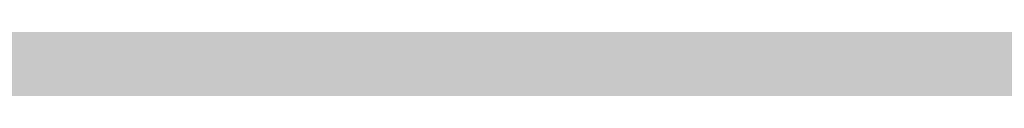
# Model space of a CAD drawing. Units: millimetres. Extents: x 0 to 2267, y 0 to 1823.
# Tile 100 of 256: x 1600.369 to 1605.705, y 1227.466 to 1227.736. Entities that reach past the tile are written whole.
import ezdxf

# ---------------------------------------------------------------- set-up
doc = ezdxf.new("R2010")
doc.units = ezdxf.units.MM
doc.header["$MEASUREMENT"] = 0
doc.layers.add('M-DIMS', color=2, linetype='Continuous', lineweight=25)
doc.layers.add('M-HATC', color=252, linetype='Continuous', lineweight=18)
doc.styles.get("Standard").update_dxf_attribs({"font": 'arial.ttf'})
doc.dimstyles.get("Standard").update_dxf_attribs({"dimtxt": 7, "dimasz": 4, "dimexe": 0.18, "dimexo": 0.0625, "dimgap": 0.09, "dimtad": 0, "dimdec": 0, "dimzin": 0, "dimdsep": 46, "dimtxsty": 'Standard', "dimcen": 0.09, "dimadec": 0, "dimazin": 0, "dimtfac": 1, "dimtdec": 0, "dimtofl": 0, "dimtmove": 0, "dimatfit": 3, "dimfxl": 1, "dimtolj": 1, "dimtzin": 0, "dimarcsym": 0})

# ---------------------------------------------------------------- blocks, each defined once
blk = doc.blocks.new('*D19')
at = {"layer": 'Defpoints', "color": 0, "transparency": 16777216}
for p in [(1605.3399, 1483.3044), (1445.5291, 1333.8851)]:
    blk.add_point(p, dxfattribs=at)
at = {"layer": 'M-DIMS', "color": 0, "lineweight": -2, "transparency": 16777216}
for p, q in [((1605.3399, 1483.2144), (1605.3399, 1483.3944)), ((1605.2499, 1483.3044), (1605.4299, 1483.3044)), ((1366.3244, 1259.8306), (1442.6072, 1331.1532))]:
    blk.add_line(p, q, dxfattribs=at)
at = {"layer": 'M-DIMS', "color": 0, "transparency": 16777216}
blk.add_solid([(1442.1519, 1331.6402), (1443.0625, 1330.6663), (1445.5291, 1333.8851)], dxfattribs=at)
at = {"layer": 'M-DIMS', "color": 0, "transparency": 16777216, "insert": (1349.6425, 1244.2335), "char_height": 7, "attachment_point": 5, "rotation": 43.0753}
blk.add_mtext('\\A1;2X R218.8', dxfattribs=at)

msp = doc.modelspace()

# ---------------------------------------------------------------- hatches: boundary and pattern name
at = {"layer": 'M-HATC'}
h = msp.add_hatch(color=256, dxfattribs=at)
h.dxf.hatch_style = 1
h.paths.add_polyline_path([(2055.771, 1603.062), (1381.0868, 1603.062), (1381.0868, 1598.062), (2055.771, 1598.062)])
h.paths.add_polyline_path([(2055.771, 1598.062), (1381.0868, 1598.062), (1381.0868, 1593.062), (2055.771, 1593.062)])
h.paths.add_polyline_path([(2051.3074, 1536.7609), (1385.5504, 1536.7609), (1385.5504, 1526.7609), (1387.5504, 1526.7609), (1388.5366, 1525.0528), (1385.3319, 1521.2335), (1385.3319, 1521.2226), (2050.2542, 1522.7491), (2048.3212, 1525.0528), (2049.3074, 1526.7609), (2051.3074, 1526.7609)])
edge = h.paths.add_edge_path()
edge.add_arc((1847.5345, 1379.1492), 135, 222.603061, 222.890851, ccw=False)
edge.add_line((1748.1663, 1287.7656), (1683.0921, 1287.7656))
edge.add_arc((1583.7239, 1379.1492), 135, 317.109149, 317.396939, ccw=False)
edge.add_arc((1678.9686, 1290.6707), 5, 222.8909, 317.1091, ccw=False)
edge.add_arc((1774.2133, 1379.1492), 135, 222.603061, 222.890851, ccw=False)
edge.add_line((1674.8451, 1287.7656), (1609.7709, 1287.7656))
edge.add_arc((1510.4027, 1379.1492), 135, 317.109149, 317.396939, ccw=False)
edge.add_arc((1605.6474, 1290.6707), 5, 222.8909, 317.1091, ccw=False)
edge.add_arc((1700.8921, 1379.1492), 135, 222.603061, 222.890851, ccw=False)
edge.add_line((1601.5239, 1287.7656), (1536.4497, 1287.7656))
edge.add_arc((1437.0815, 1379.1492), 135, 317.109149, 317.396939, ccw=False)
edge.add_arc((1532.3262, 1290.6707), 5, 222.8909, 317.1091, ccw=False)
edge.add_arc((1627.5709, 1379.1492), 135, 222.603061, 222.890851, ccw=False)
edge.add_line((1528.2027, 1287.7656), (1505.9289, 1287.7656))
edge.add_spline(control_points=[(1505.9289, 1287.7656), (1504.2622, 1287.7656), (1504.2622, 1282.7656), (1505.9289, 1282.7656)], knot_values=[0, 0, 0, 0, 5, 5, 5, 5], degree=3, periodic=0)
edge.add_line((1505.9289, 1282.7656), (1930.9289, 1282.7656))
edge.add_spline(control_points=[(1930.9289, 1282.7656), (1932.5956, 1282.7656), (1932.5956, 1287.7656), (1930.9289, 1287.7656)], knot_values=[0, 0, 0, 0, 5, 5, 5, 5], degree=3, periodic=0)
edge.add_line((1930.9289, 1287.7656), (1903.0557, 1287.7656))
edge.add_arc((1803.6875, 1379.1492), 135, 317.109149, 317.396939, ccw=False)
edge.add_arc((1898.9322, 1290.6707), 5, 222.8909, 317.1091, ccw=False)
edge.add_arc((1994.1769, 1379.1492), 135, 222.603061, 222.890851, ccw=False)
edge.add_line((1894.8087, 1287.7656), (1829.7345, 1287.7656))
edge.add_arc((1730.3663, 1379.1492), 135, 317.109149, 317.396939, ccw=False)
edge.add_arc((1825.611, 1290.6707), 5, 222.8909, 317.1091, ccw=False)
edge.add_arc((1920.8557, 1379.1492), 135, 222.603061, 222.890851, ccw=False)
edge.add_line((1821.4875, 1287.7656), (1756.4133, 1287.7656))
edge.add_arc((1657.0451, 1379.1492), 135, 317.109149, 317.396939, ccw=False)
edge.add_arc((1752.2898, 1290.6707), 5, 222.8909, 317.1091, ccw=False)
edge = h.paths.add_edge_path()
edge.add_spline(control_points=[(1843.4289, 1227.2475), (1845.0956, 1227.2475), (1845.0956, 1232.2475), (1843.4289, 1232.2475)], knot_values=[0, 0, 0, 0, 5, 5, 5, 5], degree=3, periodic=0)
edge.add_line((1843.4289, 1232.2475), (1593.4289, 1232.2475))
edge.add_spline(control_points=[(1593.4289, 1232.2475), (1591.7622, 1232.2475), (1591.7622, 1227.2475), (1593.4289, 1227.2475)], knot_values=[0, 0, 0, 0, 5, 5, 5, 5], degree=3, periodic=0)
edge.add_line((1593.4289, 1227.2475), (1843.4289, 1227.2475))
h.paths.add_polyline_path([(1905.9289, 1127.4171), (1530.9289, 1127.4171, 0.414214), (1520.9289, 1117.4171), (1530.9289, 1117.4171), (1915.9289, 1117.4171, 0.414214)])
edge = h.paths.add_edge_path()
edge.add_arc((1397.0858, 1498.4078), 12.7299, 90.78215, 190.87871, ccw=False)
edge.add_line((1396.912, 1511.1365), (1428.0097, 1511.3488))
edge.add_line((1428.0097, 1511.3488), (1433.0097, 1511.3488))
edge.add_line((1433.0097, 1511.3488), (1434.439, 1511.3488))
edge.add_arc((1419.474, 1498.0804), 20, 41.561, 74.08211)
edge.add_line((1424.9592, 1517.3135), (1399.9351, 1517.2561))
edge.add_spline(control_points=[(1399.9307, 1517.2561), (1399.884, 1517.2131), (1399.8328, 1517.1689), (1399.7774, 1517.1236)], knot_values=[11.567499, 11.567499, 11.567499, 11.567499, 11.814249, 11.814249, 11.814249, 11.814249], degree=3, periodic=0)
edge.add_spline(control_points=[(1399.6328, 1517.0099), (1399.5831, 1516.9721), (1399.5307, 1516.9338), (1399.4759, 1516.8947)], knot_values=[11.167718, 11.167718, 11.167718, 11.167718, 11.365188, 11.365188, 11.365188, 11.365188], degree=3, periodic=0)
edge.add_spline(control_points=[(1399.3398, 1516.8001), (1399.1514, 1516.6719), (1398.9384, 1516.5377), (1398.704, 1516.3994)], knot_values=[10.376405, 10.376405, 10.376405, 10.376405, 11.00994, 11.00994, 11.00994, 11.00994], degree=3, periodic=0)
edge.add_spline(control_points=[(1398.6572, 1516.3719), (1398.5789, 1516.326), (1398.4983, 1516.2797), (1398.4155, 1516.2331)], knot_values=[10.125175, 10.125175, 10.125175, 10.125175, 10.334406, 10.334406, 10.334406, 10.334406], degree=3, periodic=0)
edge.add_spline(control_points=[(1398.2642, 1516.1487), (1398.196, 1516.1111), (1398.1263, 1516.0732), (1398.0555, 1516.0351)], knot_values=[9.832246, 9.832246, 9.832246, 9.832246, 9.999658, 9.999658, 9.999658, 9.999658], degree=3, periodic=0)
edge.add_spline(control_points=[(1397.9987, 1516.0048), (1397.7312, 1515.8621), (1397.446, 1515.7171), (1397.1466, 1515.5714)], knot_values=[9.161808, 9.161808, 9.161808, 9.161808, 9.787769, 9.787769, 9.787769, 9.787769], degree=3, periodic=0)
edge.add_spline(control_points=[(1397.1466, 1515.5714), (1396.8418, 1515.423), (1396.5222, 1515.274), (1396.1914, 1515.1262)], knot_values=[8.524455, 8.524455, 8.524455, 8.524455, 9.161808, 9.161808, 9.161808, 9.161808], degree=3, periodic=0)
edge.add_spline(control_points=[(1396.0777, 1515.0756), (1395.9854, 1515.0348), (1395.8922, 1514.994), (1395.7983, 1514.9534)], knot_values=[8.275193, 8.275193, 8.275193, 8.275193, 8.451726, 8.451726, 8.451726, 8.451726], degree=3, periodic=0)
edge.add_spline(control_points=[(1395.6018, 1514.8691), (1395.4997, 1514.8257), (1395.3968, 1514.7824), (1395.2932, 1514.7394)], knot_values=[7.962917, 7.962917, 7.962917, 7.962917, 8.152764, 8.152764, 8.152764, 8.152764], degree=3, periodic=0)
edge.add_spline(control_points=[(1395.2116, 1514.7057), (1394.8278, 1514.5475), (1394.4345, 1514.3929), (1394.0364, 1514.2442)], knot_values=[7.21254, 7.21254, 7.21254, 7.21254, 7.913148, 7.913148, 7.913148, 7.913148], degree=3, periodic=0)
edge.add_spline(control_points=[(1394.0364, 1514.2442), (1393.7076, 1514.1214), (1393.3754, 1514.0027), (1393.0427, 1513.8895)], knot_values=[6.633733, 6.633733, 6.633733, 6.633733, 7.21254, 7.21254, 7.21254, 7.21254], degree=3, periodic=0)
edge.add_spline(control_points=[(1392.8214, 1513.815), (1392.7198, 1513.7812), (1392.6181, 1513.7479), (1392.5166, 1513.7152)], knot_values=[6.328796, 6.328796, 6.328796, 6.328796, 6.505493, 6.505493, 6.505493, 6.505493], degree=3, periodic=0)
edge.add_spline(control_points=[(1392.5166, 1513.7152), (1392.3187, 1513.6515), (1392.1212, 1513.59), (1391.9244, 1513.531)], knot_values=[5.984605, 5.984605, 5.984605, 5.984605, 6.328796, 6.328796, 6.328796, 6.328796], degree=3, periodic=0)
edge.add_spline(control_points=[(1391.7915, 1513.4915), (1391.3122, 1513.3501), (1390.8384, 1513.2239), (1390.3784, 1513.1171)], knot_values=[5.066697, 5.066697, 5.066697, 5.066697, 5.907055, 5.907055, 5.907055, 5.907055], degree=3, periodic=0)
edge.add_spline(control_points=[(1390.3784, 1513.1171), (1390.1797, 1513.071), (1389.9836, 1513.0284), (1389.7907, 1512.9899)], knot_values=[4.70367, 4.70367, 4.70367, 4.70367, 5.066695, 5.066695, 5.066695, 5.066695], degree=3, periodic=0)
edge.add_spline(control_points=[(1389.422, 1512.9204), (1389.2459, 1512.8892), (1389.0729, 1512.8617), (1388.9036, 1512.8381)], knot_values=[4.130571, 4.130571, 4.130571, 4.130571, 4.469816, 4.469816, 4.469816, 4.469816], degree=3, periodic=0)
edge.add_spline(control_points=[(1388.9036, 1512.8381), (1388.591, 1512.7946), (1388.2911, 1512.7644), (1388.0071, 1512.7494)], knot_values=[3.504031, 3.504031, 3.504031, 3.504031, 4.130571, 4.130571, 4.130571, 4.130571], degree=3, periodic=0)
edge.add_spline(control_points=[(1387.9356, 1512.7459), (1387.8538, 1512.7423), (1387.7733, 1512.74), (1387.6944, 1512.739)], knot_values=[3.268866, 3.268866, 3.268866, 3.268866, 3.451164, 3.451164, 3.451164, 3.451164], degree=3, periodic=0)
edge.add_spline(control_points=[(1387.3351, 1512.7443), (1387.2076, 1512.7499), (1387.0847, 1512.7597), (1386.967, 1512.7739)], knot_values=[2.670686, 2.670686, 2.670686, 2.670686, 2.984, 2.984, 2.984, 2.984], degree=3, periodic=0)
edge.add_spline(control_points=[(1386.8327, 1512.7922), (1386.8209, 1512.7941), (1386.8092, 1512.7959), (1386.7975, 1512.7979)], knot_values=[2.516981, 2.516981, 2.516981, 2.516981, 2.549528, 2.549528, 2.549528, 2.549528], degree=3, periodic=0)
edge.add_spline(control_points=[(1386.4526, 1512.8735), (1386.4257, 1512.881), (1386.3993, 1512.889), (1386.3733, 1512.8972)], knot_values=[2.095869, 2.095869, 2.095869, 2.095869, 2.17941, 2.17941, 2.17941, 2.17941], degree=3, periodic=0)
edge.add_spline(control_points=[(1386.0691, 1513.0189), (1386.0634, 1513.0217), (1386.0577, 1513.0246), (1386.052, 1513.0275)], knot_values=[1.72453, 1.72453, 1.72453, 1.72453, 1.745933, 1.745933, 1.745933, 1.745933], degree=3, periodic=0)
edge.add_arc((1399.474, 1498.0804), 20, 131.82432, 180)
edge.add_arc((1630.3336, 1505.5484), 250.9708, 181.705176, 236.427975)
edge.add_arc((1605.3399, 1483.3044), 218.7822, 238.660829, 243.34961)
edge.add_arc((1647.0911, 1510.3592), 262.8986, 183.129836, 237.853442, ccw=False)
h.paths.add_polyline_path([(1406.5369, 1391.9644, 0.149382), (1491.5506, 1296.4418, -0.129517)], flags=17)
edge = h.paths.add_edge_path()
edge.add_arc((2037.3838, 1498.0804), 20, 0, 48.26587)
edge.add_spline(control_points=[(2050.6973, 1513.0052), (2050.6512, 1512.9847), (2050.6034, 1512.9655), (2050.5539, 1512.9477)], knot_values=[1.835652, 1.835652, 1.835652, 1.835652, 2.000781, 2.000781, 2.000781, 2.000781], degree=3, periodic=0)
edge.add_spline(control_points=[(2050.4616, 1512.9166), (2050.479, 1512.9221), (2050.4963, 1512.9277), (2050.5133, 1512.9335)], knot_values=[2.045477, 2.045477, 2.045477, 2.045477, 2.101389, 2.101389, 2.101389, 2.101389], degree=3, periodic=0)
edge.add_spline(control_points=[(2050.129, 1512.8342), (2050.1984, 1512.8473), (2050.2657, 1512.8623), (2050.3308, 1512.8792)], knot_values=[2.237629, 2.237629, 2.237629, 2.237629, 2.435841, 2.435841, 2.435841, 2.435841], degree=3, periodic=0)
edge.add_spline(control_points=[(2050.0946, 1512.8278), (2050.1061, 1512.8299), (2050.1176, 1512.832), (2050.129, 1512.8342)], knot_values=[2.435841, 2.435841, 2.435841, 2.435841, 2.468321, 2.468321, 2.468321, 2.468321], degree=3, periodic=0)
edge.add_spline(control_points=[(2049.7843, 1512.7851), (2049.8552, 1512.7922), (2049.9243, 1512.8008), (2049.9917, 1512.8109)], knot_values=[2.563852, 2.563852, 2.563852, 2.563852, 2.748541, 2.748541, 2.748541, 2.748541], degree=3, periodic=0)
edge.add_spline(control_points=[(2049.4052, 1512.7617), (2049.5364, 1512.7653), (2049.6629, 1512.773), (2049.7843, 1512.7851)], knot_values=[2.748541, 2.748541, 2.748541, 2.748541, 3.064882, 3.064882, 3.064882, 3.064882], degree=3, periodic=0)
edge.add_spline(control_points=[(2049.1698, 1512.7597), (2049.2336, 1512.7591), (2049.2965, 1512.7594), (2049.3584, 1512.7606)], knot_values=[3.102309, 3.102309, 3.102309, 3.102309, 3.2503, 3.2503, 3.2503, 3.2503], degree=3, periodic=0)
edge.add_spline(control_points=[(2048.8573, 1512.7691), (2048.9638, 1512.7638), (2049.068, 1512.7606), (2049.1698, 1512.7597)], knot_values=[3.2503, 3.2503, 3.2503, 3.2503, 3.486069, 3.486069, 3.486069, 3.486069], degree=3, periodic=0)
edge.add_spline(control_points=[(2048.6924, 1512.7789), (2048.3729, 1512.8009), (2048.0345, 1512.8411), (2047.6817, 1512.897)], knot_values=[3.606429, 3.606429, 3.606429, 3.606429, 4.2989, 4.2989, 4.2989, 4.2989], degree=3, periodic=0)
edge.add_spline(control_points=[(2047.6817, 1512.897), (2047.5458, 1512.9185), (2047.4077, 1512.9424), (2047.2678, 1512.9685)], knot_values=[4.2989, 4.2989, 4.2989, 4.2989, 4.565769, 4.565769, 4.565769, 4.565769], degree=3, periodic=0)
edge.add_spline(control_points=[(2047.2678, 1512.9685), (2047.1449, 1512.9914), (2047.0207, 1513.016), (2046.8951, 1513.0422)], knot_values=[4.565769, 4.565769, 4.565769, 4.565769, 4.799971, 4.799971, 4.799971, 4.799971], degree=3, periodic=0)
edge.add_spline(control_points=[(2046.8951, 1513.0422), (2046.5286, 1513.1188), (2046.1513, 1513.209), (2045.7676, 1513.3107)], knot_values=[4.799971, 4.799971, 4.799971, 4.799971, 5.483718, 5.483718, 5.483718, 5.483718], degree=3, periodic=0)
edge.add_spline(control_points=[(2045.7676, 1513.3107), (2045.3724, 1513.4154), (2044.9704, 1513.5322), (2044.5662, 1513.6588)], knot_values=[5.483718, 5.483718, 5.483718, 5.483718, 6.187866, 6.187866, 6.187866, 6.187866], degree=3, periodic=0)
edge.add_spline(control_points=[(2044.5662, 1513.6588), (2044.4149, 1513.7061), (2044.2633, 1513.7549), (2044.1116, 1513.8048)], knot_values=[6.187866, 6.187866, 6.187866, 6.187866, 6.451551, 6.451551, 6.451551, 6.451551], degree=3, periodic=0)
edge.add_spline(control_points=[(2044.1116, 1513.8048), (2043.9967, 1513.8427), (2043.8817, 1513.8813), (2043.7668, 1513.9205)], knot_values=[6.451551, 6.451551, 6.451551, 6.451551, 6.651434, 6.651434, 6.651434, 6.651434], degree=3, periodic=0)
edge.add_spline(control_points=[(2043.7668, 1513.9205), (2043.3716, 1514.0554), (2042.9774, 1514.1979), (2042.5886, 1514.3458)], knot_values=[6.651434, 6.651434, 6.651434, 6.651434, 7.338879, 7.338879, 7.338879, 7.338879], degree=3, periodic=0)
edge.add_spline(control_points=[(2042.5886, 1514.3458), (2042.1643, 1514.5071), (2041.7465, 1514.6749), (2041.3409, 1514.846)], knot_values=[7.338879, 7.338879, 7.338879, 7.338879, 8.089209, 8.089209, 8.089209, 8.089209], degree=3, periodic=0)
edge.add_spline(control_points=[(2041.3409, 1514.846), (2041.1028, 1514.9465), (2040.869, 1515.0481), (2040.6405, 1515.1502)], knot_values=[8.089209, 8.089209, 8.089209, 8.089209, 8.529587, 8.529587, 8.529587, 8.529587], degree=3, periodic=0)
edge.add_spline(control_points=[(2040.51, 1515.2089), (2040.0824, 1515.4022), (2039.6747, 1515.5971), (2039.295, 1515.7894)], knot_values=[8.613818, 8.613818, 8.613818, 8.613818, 9.44571, 9.44571, 9.44571, 9.44571], degree=3, periodic=0)
edge.add_spline(control_points=[(2039.295, 1515.7894), (2039.0618, 1515.9075), (2038.8391, 1516.0246), (2038.6288, 1516.1398)], knot_values=[9.44571, 9.44571, 9.44571, 9.44571, 9.956404, 9.956404, 9.956404, 9.956404], degree=3, periodic=0)
edge.add_spline(control_points=[(2038.6288, 1516.1398), (2038.5187, 1516.2001), (2038.4121, 1516.2598), (2038.309, 1516.3189)], knot_values=[9.956404, 9.956404, 9.956404, 9.956404, 10.223542, 10.223542, 10.223542, 10.223542], degree=3, periodic=0)
edge.add_spline(control_points=[(2038.309, 1516.3189), (2038.2138, 1516.3735), (2038.1216, 1516.4276), (2038.0328, 1516.481)], knot_values=[10.223542, 10.223542, 10.223542, 10.223542, 10.47051, 10.47051, 10.47051, 10.47051], degree=3, periodic=0)
edge.add_spline(control_points=[(2038.0328, 1516.481), (2037.7855, 1516.6296), (2037.5639, 1516.773), (2037.3722, 1516.909)], knot_values=[10.47051, 10.47051, 10.47051, 10.47051, 11.15767, 11.15767, 11.15767, 11.15767], degree=3, periodic=0)
edge.add_spline(control_points=[(2037.3722, 1516.909), (2037.2789, 1516.9752), (2037.1927, 1517.0396), (2037.1142, 1517.102)], knot_values=[11.15767, 11.15767, 11.15767, 11.15767, 11.49227, 11.49227, 11.49227, 11.49227], degree=3, periodic=0)
edge.add_spline(control_points=[(2036.8564, 1517.3259), (2036.9148, 1517.2692), (2036.9814, 1517.2103), (2037.0557, 1517.1492)], knot_values=[11.577341, 11.577341, 11.577341, 11.577341, 11.91035, 11.91035, 11.91035, 11.91035], degree=3, periodic=0)
edge.add_spline(control_points=[(2036.8074, 1517.3748), (2036.823, 1517.3587), (2036.8393, 1517.3424), (2036.8564, 1517.3259)], knot_values=[11.91035, 11.91035, 11.91035, 11.91035, 12.007402, 12.007402, 12.007402, 12.007402], degree=3, periodic=0)
edge.add_spline(control_points=[(2036.7017, 1517.494), (2036.7104, 1517.483), (2036.7196, 1517.4719), (2036.7291, 1517.4606)], knot_values=[12.184155, 12.184155, 12.184155, 12.184155, 12.255409, 12.255409, 12.255409, 12.255409], degree=3, periodic=0)
edge.add_spline(control_points=[(2036.6159, 1517.6205), (2036.62, 1517.613), (2036.6243, 1517.6055), (2036.6289, 1517.5979)], knot_values=[12.487913, 12.487913, 12.487913, 12.487913, 12.541035, 12.541035, 12.541035, 12.541035], degree=3, periodic=0)
edge.add_spline(control_points=[(2036.5635, 1517.786), (2036.5637, 1517.7794), (2036.5642, 1517.7726), (2036.565, 1517.7658)], knot_values=[12.911761, 12.911761, 12.911761, 12.911761, 12.968286, 12.968286, 12.968286, 12.968286], degree=3, periodic=0)
edge.add_spline(control_points=[(2036.6166, 1517.9304), (2036.6125, 1517.9259), (2036.6086, 1517.9212), (2036.6049, 1517.9165)], knot_values=[13.382527, 13.382527, 13.382527, 13.382527, 13.433791, 13.433791, 13.433791, 13.433791], degree=3, periodic=0)
edge.add_spline(control_points=[(2036.749, 1518.017), (2036.7361, 1518.0116), (2036.7239, 1518.006), (2036.7124, 1518.0002)], knot_values=[13.726299, 13.726299, 13.726299, 13.726299, 13.809928, 13.809928, 13.809928, 13.809928], degree=3, periodic=0)
edge.add_spline(control_points=[(2036.8604, 1518.0528), (2036.8386, 1518.0474), (2036.8181, 1518.0416), (2036.7988, 1518.0353)], knot_values=[13.910887, 13.910887, 13.910887, 13.910887, 14.02153, 14.02153, 14.02153, 14.02153], degree=3, periodic=0)
edge.add_line((2036.9639, 1518.0804), (2032.3838, 1518.0804))
edge.add_line((2032.3838, 1518.0804), (2027.3838, 1518.0804))
edge.add_line((2027.3838, 1518.0804), (2022.3838, 1518.0804))
edge.add_line((2022.3838, 1518.0804), (2017.3838, 1518.0804))
edge.add_arc((2017.3838, 1498.0804), 20, 90, 138.439)
edge.add_line((2002.4188, 1511.3488), (2003.8481, 1511.3488))
edge.add_line((2003.8481, 1511.3488), (2008.8481, 1511.3488))
edge.add_line((2008.8481, 1511.3488), (2039.772, 1511.1377))
edge.add_arc((2039.772, 1498.4078), 12.7299, -10.87871, 90, ccw=False)
edge.add_arc((1789.7668, 1510.3592), 262.8986, 302.146558, 356.870164, ccw=False)
edge.add_arc((1831.5179, 1483.3044), 218.7822, 296.65039, 301.339171)
edge.add_arc((1806.5242, 1505.5484), 250.9708, 303.572025, 358.294824)
h.paths.add_polyline_path([(2030.321, 1391.9644, -0.129517), (1945.3072, 1296.4418, 0.149382)], flags=17)
edge = h.paths.add_edge_path()
edge.add_spline(control_points=[(2037.2464, 1518.0821), (2037.2898, 1518.081), (2037.3355, 1518.0804), (2037.3838, 1518.0804)], knot_values=[0.000012, 0.000012, 0.000012, 0.000012, 0.144754, 0.144754, 0.144754, 0.144754], degree=3, periodic=0)
edge.add_line((2037.3357, 1518.0804), (2037.0096, 1518.0804))
edge.add_spline(control_points=[(2037.0096, 1518.0804), (2036.9822, 1518.0768), (2036.956, 1518.0727), (2036.9312, 1518.0681)], knot_values=[14.13465, 14.13465, 14.13465, 14.13465, 14.247197, 14.247197, 14.247197, 14.247197], degree=3, periodic=0)
edge.add_spline(control_points=[(2036.9312, 1518.0681), (2036.9276, 1518.0674), (2036.9241, 1518.0667), (2036.9205, 1518.0661)], knot_values=[14.118315, 14.118315, 14.118315, 14.118315, 14.13465, 14.13465, 14.13465, 14.13465], degree=3, periodic=0)
edge.add_spline(control_points=[(2036.9205, 1518.0661), (2036.9118, 1518.0644), (2036.9032, 1518.0626), (2036.8948, 1518.0608)], knot_values=[14.078086, 14.078086, 14.078086, 14.078086, 14.118315, 14.118315, 14.118315, 14.118315], degree=3, periodic=0)
edge.add_spline(control_points=[(2036.8948, 1518.0608), (2036.883, 1518.0583), (2036.8716, 1518.0556), (2036.8604, 1518.0528)], knot_values=[14.02153, 14.02153, 14.02153, 14.02153, 14.078086, 14.078086, 14.078086, 14.078086], degree=3, periodic=0)
edge.add_spline(control_points=[(2036.8604, 1518.0528), (2036.8386, 1518.0474), (2036.8181, 1518.0416), (2036.7988, 1518.0353)], knot_values=[13.910887, 13.910887, 13.910887, 13.910887, 14.02153, 14.02153, 14.02153, 14.02153], degree=3, periodic=0)
edge.add_spline(control_points=[(2036.7988, 1518.0353), (2036.7981, 1518.035), (2036.7974, 1518.0348), (2036.7967, 1518.0346)], knot_values=[13.906906, 13.906906, 13.906906, 13.906906, 13.910887, 13.910887, 13.910887, 13.910887], degree=3, periodic=0)
edge.add_spline(control_points=[(2036.7967, 1518.0346), (2036.7882, 1518.0318), (2036.7799, 1518.0289), (2036.7719, 1518.0259)], knot_values=[13.857826, 13.857826, 13.857826, 13.857826, 13.906906, 13.906906, 13.906906, 13.906906], degree=3, periodic=0)
edge.add_spline(control_points=[(2036.7719, 1518.0259), (2036.764, 1518.023), (2036.7564, 1518.02), (2036.749, 1518.017)], knot_values=[13.809928, 13.809928, 13.809928, 13.809928, 13.857826, 13.857826, 13.857826, 13.857826], degree=3, periodic=0)
edge.add_spline(control_points=[(2036.749, 1518.017), (2036.7361, 1518.0116), (2036.7239, 1518.006), (2036.7124, 1518.0002)], knot_values=[13.726299, 13.726299, 13.726299, 13.726299, 13.809928, 13.809928, 13.809928, 13.809928], degree=3, periodic=0)
edge.add_spline(control_points=[(2036.7124, 1518.0002), (2036.7121, 1518), (2036.7118, 1517.9999), (2036.7115, 1517.9997)], knot_values=[13.723993, 13.723993, 13.723993, 13.723993, 13.726299, 13.726299, 13.726299, 13.726299], degree=3, periodic=0)
edge.add_spline(control_points=[(2036.7115, 1517.9997), (2036.7063, 1517.9971), (2036.7013, 1517.9944), (2036.6965, 1517.9917)], knot_values=[13.686536, 13.686536, 13.686536, 13.686536, 13.723993, 13.723993, 13.723993, 13.723993], degree=3, periodic=0)
edge.add_spline(control_points=[(2036.6965, 1517.9917), (2036.6919, 1517.9891), (2036.6874, 1517.9865), (2036.6831, 1517.9839)], knot_values=[13.651251, 13.651251, 13.651251, 13.651251, 13.686536, 13.686536, 13.686536, 13.686536], degree=3, periodic=0)
edge.add_spline(control_points=[(2036.6831, 1517.9839), (2036.6764, 1517.9798), (2036.67, 1517.9757), (2036.6639, 1517.9714)], knot_values=[13.596804, 13.596804, 13.596804, 13.596804, 13.651251, 13.651251, 13.651251, 13.651251], degree=3, periodic=0)
edge.add_spline(control_points=[(2036.6639, 1517.9714), (2036.6636, 1517.9712), (2036.6633, 1517.9709), (2036.6629, 1517.9707)], knot_values=[13.593956, 13.593956, 13.593956, 13.593956, 13.596804, 13.596804, 13.596804, 13.596804], degree=3, periodic=0)
edge.add_spline(control_points=[(2036.6629, 1517.9707), (2036.6603, 1517.9689), (2036.6577, 1517.967), (2036.6552, 1517.9651)], knot_values=[13.570322, 13.570322, 13.570322, 13.570322, 13.593956, 13.593956, 13.593956, 13.593956], degree=3, periodic=0)
edge.add_spline(control_points=[(2036.6552, 1517.9651), (2036.6525, 1517.9631), (2036.6499, 1517.9611), (2036.6474, 1517.9591)], knot_values=[13.545477, 13.545477, 13.545477, 13.545477, 13.570322, 13.570322, 13.570322, 13.570322], degree=3, periodic=0)
edge.add_spline(control_points=[(2036.6474, 1517.9591), (2036.6472, 1517.9589), (2036.6471, 1517.9588), (2036.6469, 1517.9587)], knot_values=[13.543931, 13.543931, 13.543931, 13.543931, 13.545477, 13.545477, 13.545477, 13.545477], degree=3, periodic=0)
edge.add_spline(control_points=[(2036.6469, 1517.9587), (2036.6412, 1517.9541), (2036.6358, 1517.9494), (2036.6307, 1517.9447)], knot_values=[13.488237, 13.488237, 13.488237, 13.488237, 13.543931, 13.543931, 13.543931, 13.543931], degree=3, periodic=0)
edge.add_spline(control_points=[(2036.6307, 1517.9447), (2036.6282, 1517.9423), (2036.6257, 1517.9399), (2036.6233, 1517.9374)], knot_values=[13.460307, 13.460307, 13.460307, 13.460307, 13.488237, 13.488237, 13.488237, 13.488237], degree=3, periodic=0)
edge.add_spline(control_points=[(2036.6233, 1517.9374), (2036.6215, 1517.9356), (2036.6198, 1517.9338), (2036.6181, 1517.932)], knot_values=[13.439712, 13.439712, 13.439712, 13.439712, 13.460307, 13.460307, 13.460307, 13.460307], degree=3, periodic=0)
edge.add_spline(control_points=[(2036.6181, 1517.932), (2036.6176, 1517.9315), (2036.6171, 1517.9309), (2036.6166, 1517.9304)], knot_values=[13.433791, 13.433791, 13.433791, 13.433791, 13.439712, 13.439712, 13.439712, 13.439712], degree=3, periodic=0)
edge.add_spline(control_points=[(2036.6166, 1517.9304), (2036.6125, 1517.9259), (2036.6086, 1517.9212), (2036.6049, 1517.9165)], knot_values=[13.382527, 13.382527, 13.382527, 13.382527, 13.433791, 13.433791, 13.433791, 13.433791], degree=3, periodic=0)
edge.add_spline(control_points=[(2036.6049, 1517.9165), (2036.6026, 1517.9135), (2036.6004, 1517.9104), (2036.5982, 1517.9074)], knot_values=[13.350017, 13.350017, 13.350017, 13.350017, 13.382527, 13.382527, 13.382527, 13.382527], degree=3, periodic=0)
edge.add_spline(control_points=[(2036.5982, 1517.9074), (2036.5972, 1517.9059), (2036.5962, 1517.9043), (2036.5952, 1517.9028)], knot_values=[13.333922, 13.333922, 13.333922, 13.333922, 13.350017, 13.350017, 13.350017, 13.350017], degree=3, periodic=0)
edge.add_spline(control_points=[(2036.5952, 1517.9028), (2036.5945, 1517.9018), (2036.5939, 1517.9009), (2036.5933, 1517.8999)], knot_values=[13.323828, 13.323828, 13.323828, 13.323828, 13.333922, 13.333922, 13.333922, 13.333922], degree=3, periodic=0)
edge.add_spline(control_points=[(2036.5933, 1517.8999), (2036.5905, 1517.8955), (2036.5879, 1517.8909), (2036.5855, 1517.8864)], knot_values=[13.277545, 13.277545, 13.277545, 13.277545, 13.323828, 13.323828, 13.323828, 13.323828], degree=3, periodic=0)
edge.add_spline(control_points=[(2036.5855, 1517.8864), (2036.5836, 1517.8827), (2036.5817, 1517.8789), (2036.5801, 1517.8751)], knot_values=[13.240119, 13.240119, 13.240119, 13.240119, 13.277545, 13.277545, 13.277545, 13.277545], degree=3, periodic=0)
edge.add_spline(control_points=[(2036.5801, 1517.8751), (2036.5795, 1517.8739), (2036.579, 1517.8727), (2036.5785, 1517.8715)], knot_values=[13.228211, 13.228211, 13.228211, 13.228211, 13.240119, 13.240119, 13.240119, 13.240119], degree=3, periodic=0)
edge.add_spline(control_points=[(2036.5785, 1517.8715), (2036.578, 1517.8702), (2036.5774, 1517.869), (2036.5769, 1517.8677)], knot_values=[13.215717, 13.215717, 13.215717, 13.215717, 13.228211, 13.228211, 13.228211, 13.228211], degree=3, periodic=0)
edge.add_spline(control_points=[(2036.5769, 1517.8677), (2036.5755, 1517.864), (2036.5741, 1517.8603), (2036.5729, 1517.8565)], knot_values=[13.179847, 13.179847, 13.179847, 13.179847, 13.215717, 13.215717, 13.215717, 13.215717], degree=3, periodic=0)
edge.add_spline(control_points=[(2036.5729, 1517.8565), (2036.5713, 1517.8515), (2036.5699, 1517.8464), (2036.5687, 1517.8413)], knot_values=[13.132017, 13.132017, 13.132017, 13.132017, 13.179847, 13.179847, 13.179847, 13.179847], degree=3, periodic=0)
edge.add_spline(control_points=[(2036.5687, 1517.8413), (2036.5684, 1517.8402), (2036.5682, 1517.8392), (2036.568, 1517.8382)], knot_values=[13.122482, 13.122482, 13.122482, 13.122482, 13.132017, 13.132017, 13.132017, 13.132017], degree=3, periodic=0)
edge.add_spline(control_points=[(2036.568, 1517.8382), (2036.5676, 1517.8363), (2036.5672, 1517.8345), (2036.5669, 1517.8327)], knot_values=[13.105592, 13.105592, 13.105592, 13.105592, 13.122482, 13.122482, 13.122482, 13.122482], degree=3, periodic=0)
edge.add_spline(control_points=[(2036.5669, 1517.8327), (2036.5662, 1517.8292), (2036.5657, 1517.8257), (2036.5652, 1517.8222)], knot_values=[13.074063, 13.074063, 13.074063, 13.074063, 13.105592, 13.105592, 13.105592, 13.105592], degree=3, periodic=0)
edge.add_spline(control_points=[(2036.5652, 1517.8222), (2036.5652, 1517.8222), (2036.5652, 1517.8222), (2036.5652, 1517.8222)], knot_values=[13.074043, 13.074043, 13.074043, 13.074043, 13.074063, 13.074063, 13.074063, 13.074063], degree=3, periodic=0)
edge.add_spline(control_points=[(2036.5652, 1517.8222), (2036.5644, 1517.8164), (2036.5639, 1517.8106), (2036.5636, 1517.8046)], knot_values=[13.021884, 13.021884, 13.021884, 13.021884, 13.074043, 13.074043, 13.074043, 13.074043], degree=3, periodic=0)
edge.add_spline(control_points=[(2036.5636, 1517.8046), (2036.5636, 1517.804), (2036.5636, 1517.8034), (2036.5635, 1517.8028)], knot_values=[13.01674, 13.01674, 13.01674, 13.01674, 13.021884, 13.021884, 13.021884, 13.021884], degree=3, periodic=0)
edge.add_spline(control_points=[(2036.5635, 1517.8028), (2036.5634, 1517.8005), (2036.5634, 1517.7982), (2036.5634, 1517.7958)], knot_values=[12.996438, 12.996438, 12.996438, 12.996438, 13.01674, 13.01674, 13.01674, 13.01674], degree=3, periodic=0)
edge.add_spline(control_points=[(2036.5634, 1517.7958), (2036.5633, 1517.7926), (2036.5634, 1517.7893), (2036.5635, 1517.786)], knot_values=[12.968286, 12.968286, 12.968286, 12.968286, 12.996438, 12.996438, 12.996438, 12.996438], degree=3, periodic=0)
edge.add_spline(control_points=[(2036.5635, 1517.786), (2036.5637, 1517.7794), (2036.5642, 1517.7726), (2036.565, 1517.7658)], knot_values=[12.911761, 12.911761, 12.911761, 12.911761, 12.968286, 12.968286, 12.968286, 12.968286], degree=3, periodic=0)
edge.add_spline(control_points=[(2036.565, 1517.7658), (2036.565, 1517.7657), (2036.565, 1517.7656), (2036.565, 1517.7656)], knot_values=[12.911017, 12.911017, 12.911017, 12.911017, 12.911761, 12.911761, 12.911761, 12.911761], degree=3, periodic=0)
edge.add_spline(control_points=[(2036.565, 1517.7656), (2036.5654, 1517.7625), (2036.5658, 1517.7593), (2036.5663, 1517.7562)], knot_values=[12.88528, 12.88528, 12.88528, 12.88528, 12.911017, 12.911017, 12.911017, 12.911017], degree=3, periodic=0)
edge.add_spline(control_points=[(2036.5663, 1517.7562), (2036.5667, 1517.7534), (2036.5672, 1517.7506), (2036.5677, 1517.7478)], knot_values=[12.862519, 12.862519, 12.862519, 12.862519, 12.88528, 12.88528, 12.88528, 12.88528], degree=3, periodic=0)
edge.add_spline(control_points=[(2036.5677, 1517.7478), (2036.5678, 1517.7474), (2036.5679, 1517.7469), (2036.568, 1517.7465)], knot_values=[12.858885, 12.858885, 12.858885, 12.858885, 12.862519, 12.862519, 12.862519, 12.862519], degree=3, periodic=0)
edge.add_spline(control_points=[(2036.568, 1517.7465), (2036.5692, 1517.7399), (2036.5707, 1517.7332), (2036.5724, 1517.7264)], knot_values=[12.8053, 12.8053, 12.8053, 12.8053, 12.858885, 12.858885, 12.858885, 12.858885], degree=3, periodic=0)
edge.add_spline(control_points=[(2036.5724, 1517.7264), (2036.5734, 1517.7226), (2036.5745, 1517.7187), (2036.5756, 1517.7149)], knot_values=[12.775176, 12.775176, 12.775176, 12.775176, 12.8053, 12.8053, 12.8053, 12.8053], degree=3, periodic=0)
edge.add_spline(control_points=[(2036.5756, 1517.7149), (2036.5763, 1517.7125), (2036.577, 1517.7102), (2036.5778, 1517.7078)], knot_values=[12.756759, 12.756759, 12.756759, 12.756759, 12.775176, 12.775176, 12.775176, 12.775176], degree=3, periodic=0)
edge.add_spline(control_points=[(2036.5778, 1517.7078), (2036.5781, 1517.7067), (2036.5784, 1517.7057), (2036.5787, 1517.7047)], knot_values=[12.748742, 12.748742, 12.748742, 12.748742, 12.756759, 12.756759, 12.756759, 12.756759], degree=3, periodic=0)
edge.add_spline(control_points=[(2036.5787, 1517.7047), (2036.5808, 1517.6983), (2036.5831, 1517.6919), (2036.5856, 1517.6854)], knot_values=[12.69959, 12.69959, 12.69959, 12.69959, 12.748742, 12.748742, 12.748742, 12.748742], degree=3, periodic=0)
edge.add_spline(control_points=[(2036.5856, 1517.6854), (2036.5876, 1517.68), (2036.5898, 1517.6746), (2036.5921, 1517.6692)], knot_values=[12.659038, 12.659038, 12.659038, 12.659038, 12.69959, 12.69959, 12.69959, 12.69959], degree=3, periodic=0)
edge.add_spline(control_points=[(2036.5921, 1517.6692), (2036.594, 1517.6648), (2036.5959, 1517.6605), (2036.5979, 1517.6561)], knot_values=[12.626806, 12.626806, 12.626806, 12.626806, 12.659038, 12.659038, 12.659038, 12.659038], degree=3, periodic=0)
edge.add_spline(control_points=[(2036.5979, 1517.6561), (2036.5984, 1517.6551), (2036.5989, 1517.6541), (2036.5993, 1517.6531)], knot_values=[12.619394, 12.619394, 12.619394, 12.619394, 12.626806, 12.626806, 12.626806, 12.626806], degree=3, periodic=0)
edge.add_spline(control_points=[(2036.5993, 1517.6531), (2036.6043, 1517.6424), (2036.6099, 1517.6315), (2036.6159, 1517.6205)], knot_values=[12.541039, 12.541039, 12.541039, 12.541039, 12.619394, 12.619394, 12.619394, 12.619394], degree=3, periodic=0)
edge.add_spline(control_points=[(2036.6159, 1517.6205), (2036.6159, 1517.6205), (2036.6159, 1517.6205), (2036.6159, 1517.6205)], knot_values=[12.541035, 12.541035, 12.541035, 12.541035, 12.541039, 12.541039, 12.541039, 12.541039], degree=3, periodic=0)
edge.add_spline(control_points=[(2036.6159, 1517.6205), (2036.62, 1517.613), (2036.6243, 1517.6055), (2036.6289, 1517.5979)], knot_values=[12.487913, 12.487913, 12.487913, 12.487913, 12.541035, 12.541035, 12.541035, 12.541035], degree=3, periodic=0)
edge.add_spline(control_points=[(2036.6289, 1517.5979), (2036.6326, 1517.5916), (2036.6365, 1517.5853), (2036.6406, 1517.5789)], knot_values=[12.443982, 12.443982, 12.443982, 12.443982, 12.487913, 12.487913, 12.487913, 12.487913], degree=3, periodic=0)
edge.add_spline(control_points=[(2036.6406, 1517.5789), (2036.6414, 1517.5776), (2036.6423, 1517.5763), (2036.6431, 1517.5749)], knot_values=[12.434996, 12.434996, 12.434996, 12.434996, 12.443982, 12.443982, 12.443982, 12.443982], degree=3, periodic=0)
edge.add_spline(control_points=[(2036.6431, 1517.5749), (2036.6531, 1517.5596), (2036.6639, 1517.5439), (2036.6756, 1517.528)], knot_values=[12.329647, 12.329647, 12.329647, 12.329647, 12.434996, 12.434996, 12.434996, 12.434996], degree=3, periodic=0)
edge.add_spline(control_points=[(2036.6756, 1517.528), (2036.6839, 1517.5168), (2036.6925, 1517.5055), (2036.7017, 1517.494)], knot_values=[12.255409, 12.255409, 12.255409, 12.255409, 12.329647, 12.329647, 12.329647, 12.329647], degree=3, periodic=0)
edge.add_spline(control_points=[(2036.7017, 1517.494), (2036.7104, 1517.483), (2036.7196, 1517.4719), (2036.7291, 1517.4606)], knot_values=[12.184155, 12.184155, 12.184155, 12.184155, 12.255409, 12.255409, 12.255409, 12.255409], degree=3, periodic=0)
edge.add_spline(control_points=[(2036.7291, 1517.4606), (2036.7436, 1517.4435), (2036.759, 1517.4262), (2036.7753, 1517.4085)], knot_values=[12.075961, 12.075961, 12.075961, 12.075961, 12.184155, 12.184155, 12.184155, 12.184155], degree=3, periodic=0)
edge.add_spline(control_points=[(2036.7753, 1517.4085), (2036.7763, 1517.4075), (2036.7773, 1517.4064), (2036.7783, 1517.4054)], knot_values=[12.069502, 12.069502, 12.069502, 12.069502, 12.075961, 12.075961, 12.075961, 12.075961], degree=3, periodic=0)
edge.add_spline(control_points=[(2036.7783, 1517.4054), (2036.7877, 1517.3953), (2036.7974, 1517.385), (2036.8074, 1517.3748)], knot_values=[12.007402, 12.007402, 12.007402, 12.007402, 12.069502, 12.069502, 12.069502, 12.069502], degree=3, periodic=0)
edge.add_spline(control_points=[(2036.8074, 1517.3748), (2036.823, 1517.3587), (2036.8393, 1517.3424), (2036.8564, 1517.3259)], knot_values=[11.91035, 11.91035, 11.91035, 11.91035, 12.007402, 12.007402, 12.007402, 12.007402], degree=3, periodic=0)
edge.add_spline(control_points=[(2036.8564, 1517.3259), (2036.9148, 1517.2692), (2036.9814, 1517.2103), (2037.0557, 1517.1492)], knot_values=[11.577341, 11.577341, 11.577341, 11.577341, 11.91035, 11.91035, 11.91035, 11.91035], degree=3, periodic=0)
edge.add_spline(control_points=[(2037.0557, 1517.1492), (2037.0747, 1517.1336), (2037.0942, 1517.1179), (2037.1142, 1517.102)], knot_values=[11.49227, 11.49227, 11.49227, 11.49227, 11.577341, 11.577341, 11.577341, 11.577341], degree=3, periodic=0)
edge.add_spline(control_points=[(2037.1142, 1517.102), (2037.1927, 1517.0396), (2037.2789, 1516.9752), (2037.3722, 1516.909)], knot_values=[11.15767, 11.15767, 11.15767, 11.15767, 11.49227, 11.49227, 11.49227, 11.49227], degree=3, periodic=0)
edge.add_spline(control_points=[(2037.3722, 1516.909), (2037.5639, 1516.773), (2037.7855, 1516.6296), (2038.0328, 1516.481)], knot_values=[10.47051, 10.47051, 10.47051, 10.47051, 11.15767, 11.15767, 11.15767, 11.15767], degree=3, periodic=0)
edge.add_spline(control_points=[(2038.0328, 1516.481), (2038.1216, 1516.4276), (2038.2138, 1516.3735), (2038.309, 1516.3189)], knot_values=[10.223542, 10.223542, 10.223542, 10.223542, 10.47051, 10.47051, 10.47051, 10.47051], degree=3, periodic=0)
edge.add_spline(control_points=[(2038.309, 1516.3189), (2038.4121, 1516.2598), (2038.5187, 1516.2001), (2038.6288, 1516.1398)], knot_values=[9.956404, 9.956404, 9.956404, 9.956404, 10.223542, 10.223542, 10.223542, 10.223542], degree=3, periodic=0)
edge.add_spline(control_points=[(2038.6288, 1516.1398), (2038.8391, 1516.0246), (2039.0618, 1515.9075), (2039.295, 1515.7894)], knot_values=[9.44571, 9.44571, 9.44571, 9.44571, 9.956404, 9.956404, 9.956404, 9.956404], degree=3, periodic=0)
edge.add_spline(control_points=[(2039.295, 1515.7894), (2039.6747, 1515.5971), (2040.0824, 1515.4022), (2040.51, 1515.2089)], knot_values=[8.613818, 8.613818, 8.613818, 8.613818, 9.44571, 9.44571, 9.44571, 9.44571], degree=3, periodic=0)
edge.add_spline(control_points=[(2040.51, 1515.2089), (2040.5533, 1515.1893), (2040.5968, 1515.1697), (2040.6405, 1515.1502)], knot_values=[8.529587, 8.529587, 8.529587, 8.529587, 8.613818, 8.613818, 8.613818, 8.613818], degree=3, periodic=0)
edge.add_spline(control_points=[(2040.6405, 1515.1502), (2040.869, 1515.0481), (2041.1028, 1514.9465), (2041.3409, 1514.846)], knot_values=[8.089209, 8.089209, 8.089209, 8.089209, 8.529587, 8.529587, 8.529587, 8.529587], degree=3, periodic=0)
edge.add_spline(control_points=[(2041.3409, 1514.846), (2041.7465, 1514.6749), (2042.1643, 1514.5071), (2042.5886, 1514.3458)], knot_values=[7.338879, 7.338879, 7.338879, 7.338879, 8.089209, 8.089209, 8.089209, 8.089209], degree=3, periodic=0)
edge.add_spline(control_points=[(2042.5886, 1514.3458), (2042.9774, 1514.1979), (2043.3716, 1514.0554), (2043.7668, 1513.9205)], knot_values=[6.651434, 6.651434, 6.651434, 6.651434, 7.338879, 7.338879, 7.338879, 7.338879], degree=3, periodic=0)
edge.add_spline(control_points=[(2043.7668, 1513.9205), (2043.8817, 1513.8813), (2043.9967, 1513.8427), (2044.1116, 1513.8048)], knot_values=[6.451551, 6.451551, 6.451551, 6.451551, 6.651434, 6.651434, 6.651434, 6.651434], degree=3, periodic=0)
edge.add_spline(control_points=[(2044.1116, 1513.8048), (2044.2633, 1513.7549), (2044.4149, 1513.7061), (2044.5662, 1513.6588)], knot_values=[6.187866, 6.187866, 6.187866, 6.187866, 6.451551, 6.451551, 6.451551, 6.451551], degree=3, periodic=0)
edge.add_spline(control_points=[(2044.5662, 1513.6588), (2044.9704, 1513.5322), (2045.3724, 1513.4154), (2045.7676, 1513.3107)], knot_values=[5.483718, 5.483718, 5.483718, 5.483718, 6.187866, 6.187866, 6.187866, 6.187866], degree=3, periodic=0)
edge.add_spline(control_points=[(2045.7676, 1513.3107), (2046.1513, 1513.209), (2046.5286, 1513.1188), (2046.8951, 1513.0422)], knot_values=[4.799971, 4.799971, 4.799971, 4.799971, 5.483718, 5.483718, 5.483718, 5.483718], degree=3, periodic=0)
edge.add_spline(control_points=[(2046.8951, 1513.0422), (2047.0207, 1513.016), (2047.1449, 1512.9914), (2047.2678, 1512.9685)], knot_values=[4.565769, 4.565769, 4.565769, 4.565769, 4.799971, 4.799971, 4.799971, 4.799971], degree=3, periodic=0)
edge.add_spline(control_points=[(2047.2678, 1512.9685), (2047.4077, 1512.9424), (2047.5458, 1512.9185), (2047.6817, 1512.897)], knot_values=[4.2989, 4.2989, 4.2989, 4.2989, 4.565769, 4.565769, 4.565769, 4.565769], degree=3, periodic=0)
edge.add_spline(control_points=[(2047.6817, 1512.897), (2048.0345, 1512.8411), (2048.3729, 1512.8009), (2048.6924, 1512.7789)], knot_values=[3.606429, 3.606429, 3.606429, 3.606429, 4.2989, 4.2989, 4.2989, 4.2989], degree=3, periodic=0)
edge.add_spline(control_points=[(2048.6924, 1512.7789), (2048.7479, 1512.7751), (2048.8029, 1512.7718), (2048.8573, 1512.7691)], knot_values=[3.486069, 3.486069, 3.486069, 3.486069, 3.606429, 3.606429, 3.606429, 3.606429], degree=3, periodic=0)
edge.add_spline(control_points=[(2048.8573, 1512.7691), (2048.9638, 1512.7638), (2049.068, 1512.7606), (2049.1698, 1512.7597)], knot_values=[3.2503, 3.2503, 3.2503, 3.2503, 3.486069, 3.486069, 3.486069, 3.486069], degree=3, periodic=0)
edge.add_spline(control_points=[(2049.1698, 1512.7597), (2049.2336, 1512.7591), (2049.2965, 1512.7594), (2049.3584, 1512.7606)], knot_values=[3.102309, 3.102309, 3.102309, 3.102309, 3.2503, 3.2503, 3.2503, 3.2503], degree=3, periodic=0)
edge.add_spline(control_points=[(2049.3584, 1512.7606), (2049.3741, 1512.7609), (2049.3897, 1512.7613), (2049.4052, 1512.7617)], knot_values=[3.064882, 3.064882, 3.064882, 3.064882, 3.102309, 3.102309, 3.102309, 3.102309], degree=3, periodic=0)
edge.add_spline(control_points=[(2049.4052, 1512.7617), (2049.5364, 1512.7653), (2049.6629, 1512.773), (2049.7843, 1512.7851)], knot_values=[2.748541, 2.748541, 2.748541, 2.748541, 3.064882, 3.064882, 3.064882, 3.064882], degree=3, periodic=0)
edge.add_spline(control_points=[(2049.7843, 1512.7851), (2049.8552, 1512.7922), (2049.9243, 1512.8008), (2049.9917, 1512.8109)], knot_values=[2.563852, 2.563852, 2.563852, 2.563852, 2.748541, 2.748541, 2.748541, 2.748541], degree=3, periodic=0)
edge.add_spline(control_points=[(2049.9917, 1512.8109), (2050.0265, 1512.8161), (2050.0608, 1512.8218), (2050.0946, 1512.8278)], knot_values=[2.468321, 2.468321, 2.468321, 2.468321, 2.563852, 2.563852, 2.563852, 2.563852], degree=3, periodic=0)
edge.add_spline(control_points=[(2050.0946, 1512.8278), (2050.1061, 1512.8299), (2050.1176, 1512.832), (2050.129, 1512.8342)], knot_values=[2.435841, 2.435841, 2.435841, 2.435841, 2.468321, 2.468321, 2.468321, 2.468321], degree=3, periodic=0)
edge.add_spline(control_points=[(2050.129, 1512.8342), (2050.1984, 1512.8473), (2050.2657, 1512.8623), (2050.3308, 1512.8792)], knot_values=[2.237629, 2.237629, 2.237629, 2.237629, 2.435841, 2.435841, 2.435841, 2.435841], degree=3, periodic=0)
edge.add_spline(control_points=[(2050.3308, 1512.8792), (2050.3754, 1512.8908), (2050.4191, 1512.9032), (2050.4616, 1512.9166)], knot_values=[2.101389, 2.101389, 2.101389, 2.101389, 2.237629, 2.237629, 2.237629, 2.237629], degree=3, periodic=0)
edge.add_spline(control_points=[(2050.4616, 1512.9166), (2050.479, 1512.9221), (2050.4963, 1512.9277), (2050.5133, 1512.9335)], knot_values=[2.045477, 2.045477, 2.045477, 2.045477, 2.101389, 2.101389, 2.101389, 2.101389], degree=3, periodic=0)
edge.add_spline(control_points=[(2050.5133, 1512.9335), (2050.527, 1512.9382), (2050.5405, 1512.9429), (2050.5539, 1512.9477)], knot_values=[2.000781, 2.000781, 2.000781, 2.000781, 2.045477, 2.045477, 2.045477, 2.045477], degree=3, periodic=0)
edge.add_spline(control_points=[(2050.5539, 1512.9477), (2050.6034, 1512.9655), (2050.6512, 1512.9847), (2050.6973, 1513.0052)], knot_values=[1.835652, 1.835652, 1.835652, 1.835652, 2.000781, 2.000781, 2.000781, 2.000781], degree=3, periodic=0)
edge.add_arc((2037.3838, 1498.0804), 20, 48.26587, 90.12993)
edge = h.paths.add_edge_path(flags=16)
edge.add_spline(control_points=[(1386.1389, 1512.9859), (1388.92, 1511.7395), (1398.0387, 1515.5187), (1399.9307, 1517.2561)], knot_values=[1.831046, 1.831046, 1.831046, 1.831046, 11.814249, 11.814249, 11.814249, 11.814249], degree=3, periodic=0)
edge.add_line((1399.9307, 1517.2561), (1393.7435, 1517.2419))
edge.add_arc((1399.474, 1498.0804), 20, 106.6501, 131.8173)

# ---------------------------------------------------------------- dimensions: what is measured, and where the dimension line sits
at = {"layer": 'M-DIMS'}
dim = msp.add_radius_dim(center=(1605.3399, 1483.3044), mpoint=(1445.5291, 1333.8851), text='2X <>', dimstyle='Standard', override={"dimdec": 1, "dimlfac": 1, "dimrnd": 0, "dimzin": 0, "dimdsep": 46, "dimlunit": 2}, dxfattribs=at)
dim.commit()
dim.dimension.update_dxf_attribs({"geometry": '*D19', "text_midpoint": (1349.6425, 1244.2335), "dimtype": 164})

doc.saveas('drawing.dxf')
